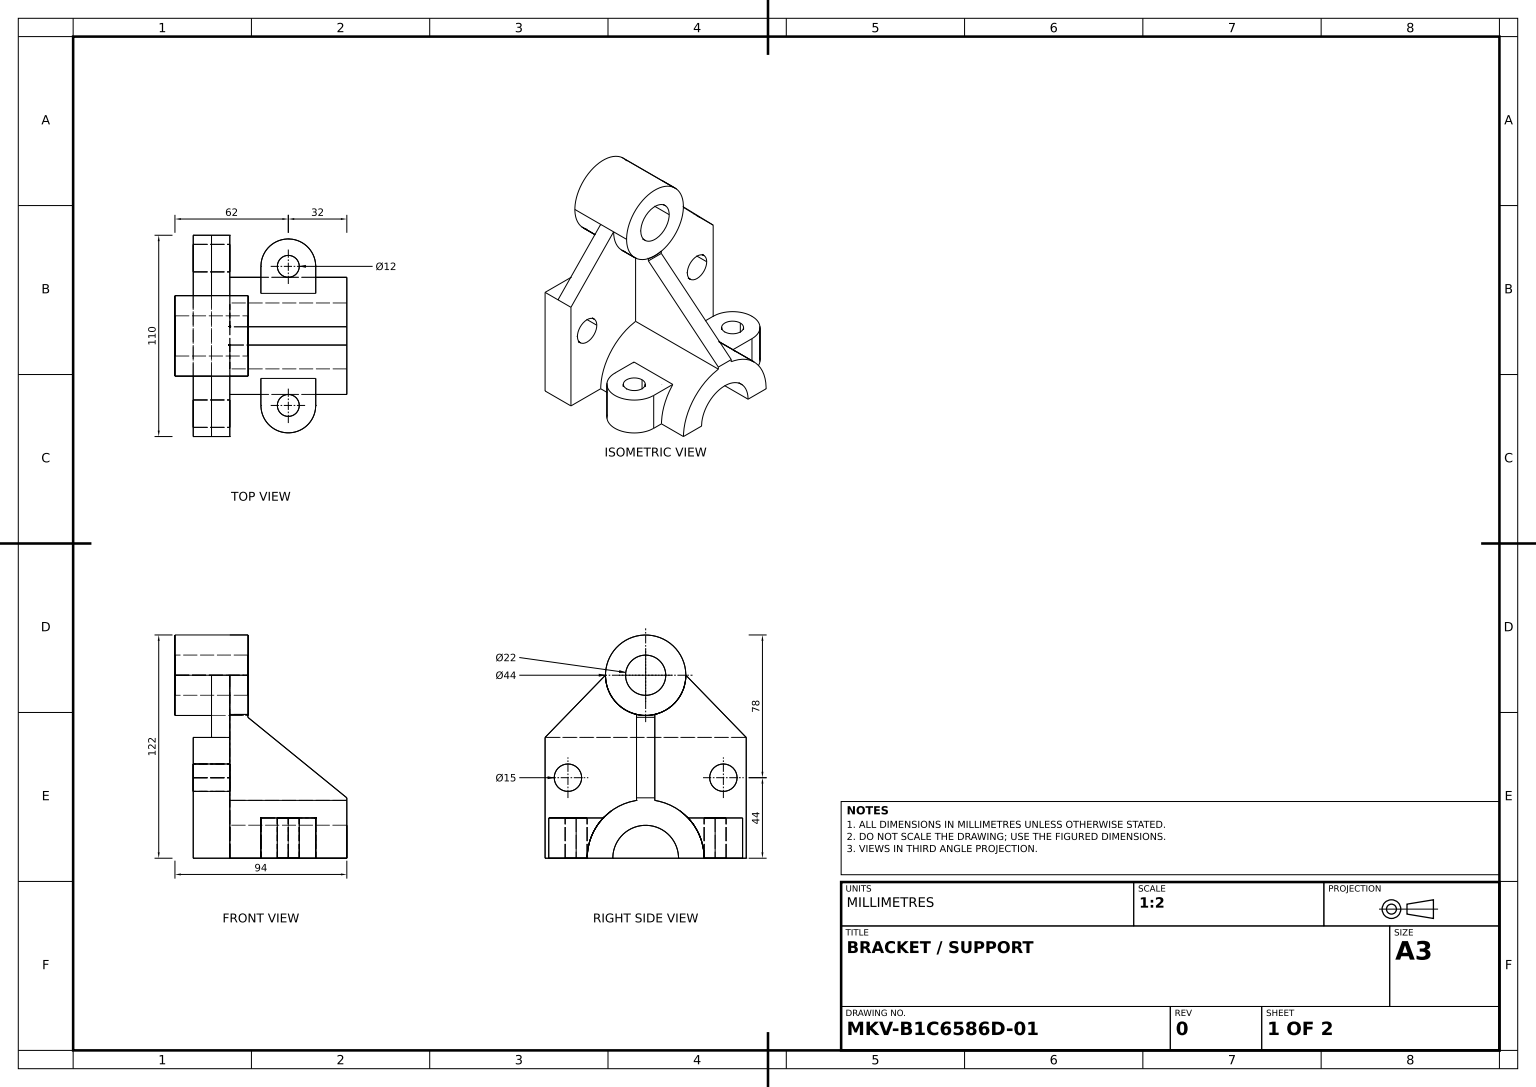
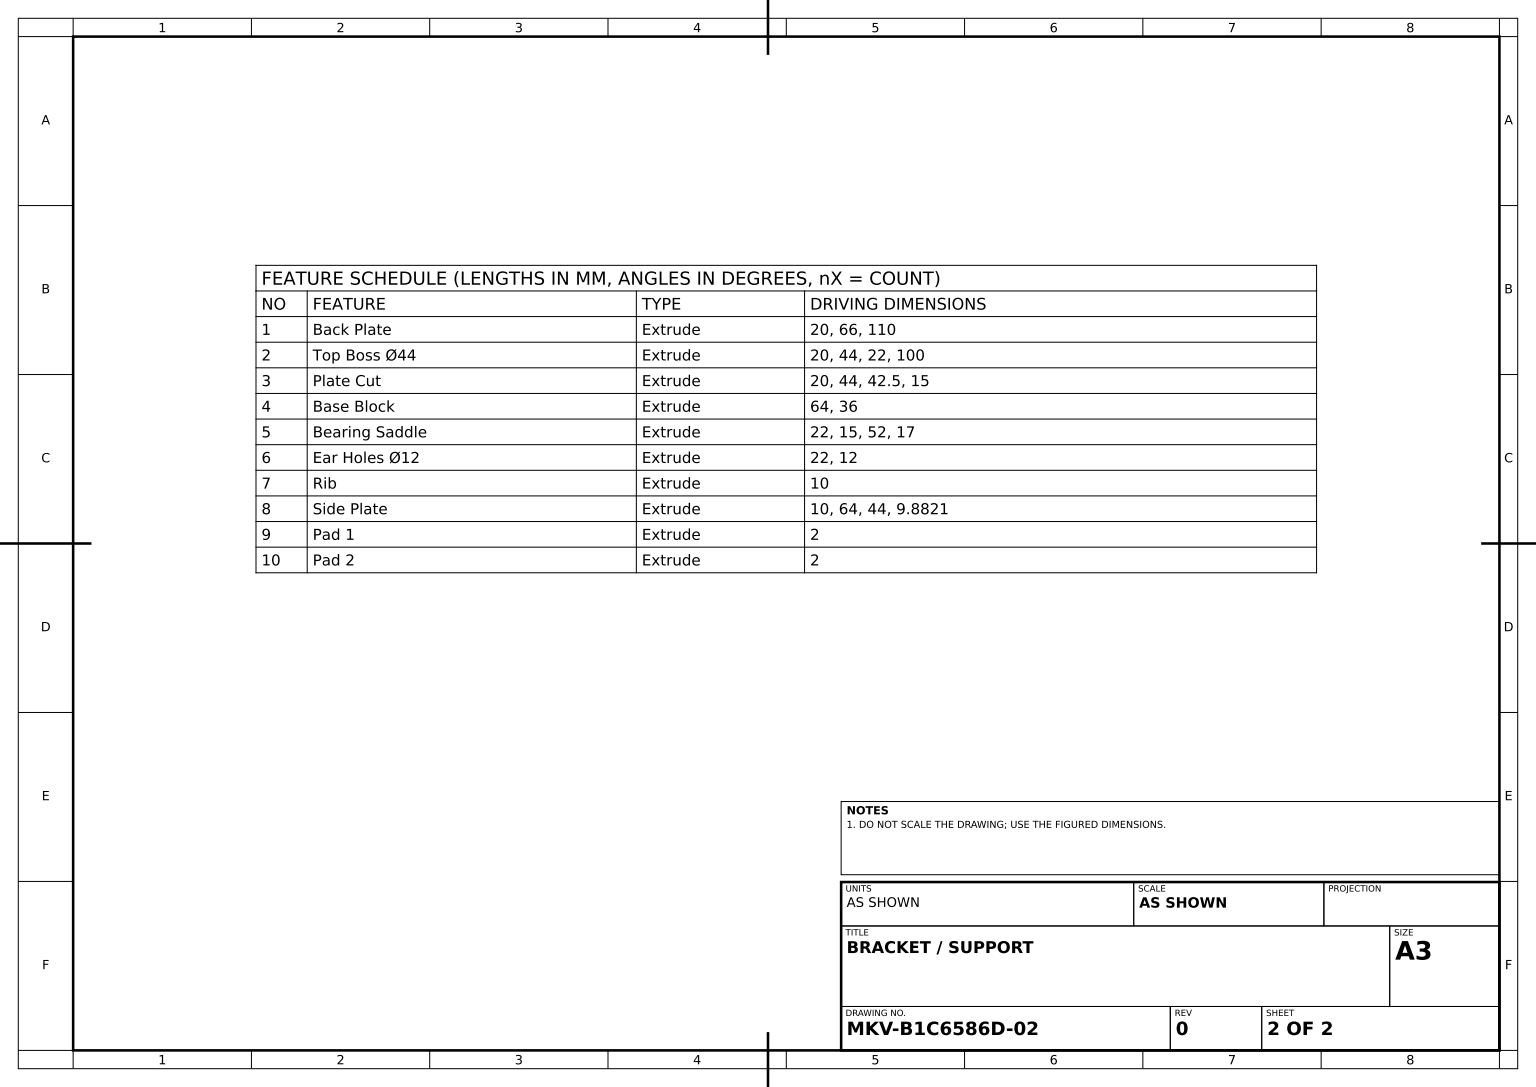
SolidWorks part; units mm, degrees
material "Plain Carbon Steel"
ref_plane "Front Plane" through (0, 0, 0) normal (0, 0, 1) x (1, 0, 0)
ref_plane "Top Plane" through (0, 0, 0) normal (0, 1, 0) x (1, 0, 0)
ref_plane "Right Plane" through (0, 0, 0) normal (1, 0, 0) x (0, 0, -1)
sketch "Back Plate Sketch" plane through (0, 0, 0) normal (1, 0, 0) x (0, 0, -1)
  line L1 (-55, 33) -> (55, 33)
  line L2 (-55, 33) -> (-55, -33)
  line L3 (-55, -33) -> (55, -33)
  line L4 (55, 33) -> (55, -33)
  line L5 (-55, 33) -> (55, -33) construction
  line L6 (-55, -33) -> (55, 33) construction
  point P0 (0, 0)
  dimension "D1" = 66
  dimension "D2" = 110
extrude "Back Plate" add sketch "Back Plate Sketch" along normal mid plane 20
sketch "Top Boss Sketch" plane through (0, 0, 0) normal (1, 0, 0) x (0, 0, -1)
  line L0 (0, -33) -> (0, 67) construction
  line L1 (-55, -33) -> (55, -33) construction
  circle A0 centre (0, 67) radius 22
  circle A1 centre (0, 67) radius 11
  dimension "D1" = 44
  dimension "D2" = 44
  dimension "D3" = 22
  dimension "D4" = 100
extrude "Top Boss Ø44" add sketch "Top Boss Sketch" along normal blind 20 and the other way blind 20 separate body
sketch "Plate Cut Sketch" plane through (10, 0, 0) normal (1, 0, 0) x (0, 0, -1)
  line L0 (0, -33) -> (0, 11) construction
  line L1 (-55, -33) -> (55, -33) construction
  line L2 (0, 11) -> (42.5, 11) construction
  circle A0 centre (42.5, 11) radius 7.5
  circle A1 centre (-42.5, 11) radius 7.5
  dimension "D3" = 15
  dimension "D1" = 44
  dimension "D2" = 42.5
extrude "Plate Cut" cut sketch "Plate Cut Sketch" against normal blind 20
sketch "Base Block Sketch" plane through (10, 0, 0) normal (1, 0, 0) x (0, 0, -1)
  line L0 (-55, -33) -> (55, -33) construction
  line L1 (-32, -33) -> (-18, -33)
  line L2 (18, -33) -> (32, -33)
  arc A0 (32, -33) -> (-32, -33) centre (0, -33) ccw
  arc A1 (18, -33) -> (-18, -33) centre (0, -33) ccw
  dimension "D1" = 64
  dimension "D2" = 36
extrude "Base Block" add sketch "Base Block Sketch" along normal blind 64
sketch "Bearing Saddle Sketch" plane through (0, -33, 0) normal (0, -1, 0) x (1, 0, 0)
  line L0 (42, 38) -> (42, -45.3499) construction
  line L1 (-10, 55) -> (-10, -55) construction
  line L2 (0, 0) -> (88.1033, 0) construction
  line L3 (27, 38) -> (27, 18)
  line L4 (74, 18) -> (10, 18) construction
  line L5 (27, 18) -> (57, 18)
  line L6 (57, 18) -> (57, 38)
  line L7 (27, -38) -> (27, -18)
  line L8 (27, -18) -> (57, -18)
  line L9 (57, -18) -> (57, -38)
  line L10 (10, -55) -> (-10, -55) construction
  arc A3 (27, 38) -> (57, 38) centre (42, 38) cw
  arc A4 (27, -38) -> (57, -38) centre (42, -38) ccw
  dimension "D1" = 15
  dimension "D2" = 52
  dimension "D3" = 17
extrude "Bearing Saddle" add sketch "Bearing Saddle Sketch" against normal blind 22
sketch "Ear Holes Sketch" plane through (0, -11, 0) normal (0, 1, 0) x (1, 0, 0)
  circle A0 centre (42, 38) radius 6
  circle A1 centre (42, -38) radius 6
  dimension "D1" = 12
extrude "Ear Holes Ø12" cut sketch "Ear Holes Sketch" against normal blind 22
sketch "Rib Sketch" plane through (10, 0, 0) normal (1, 0, 0) x (0, 0, -1)
  line L0 (-47.4205, 67) -> (37.9135, 67) construction
  line L1 (-22, 67) -> (-55, 33)
  line L2 (55, 33) -> (22, 67)
  line L5 (32, -33) -> (55, -33)
  line L6 (55, -33) -> (55, 33)
  line L7 (55, 33) -> (-55, 33)
  line L8 (-55, 33) -> (-55, -33)
  line L9 (-55, -33) -> (-32, -33)
  line L12 (55, 33) -> (-55, 33)
  circle A0 centre (0, 67) radius 22 construction
  arc A1 (32, -33) -> (-32, -33) centre (0, -33) ccw
  arc A3 (-22, 67) -> (22, 67) centre (0, 67) ccw
  dimension "D1" = 0
extrude "Rib" add sketch "Rib Sketch" against normal blind 10
sketch "Side Plate Sketch" plane through (0, 0, 0) normal (0, 0, 1) x (1, 0, 0)
  line L1 (10, 44) -> (19.8821, 44)
  line L2 (10, 67) -> (10, 33) construction
  line L3 (10, 44) -> (10, 0)
  line L4 (10, 33) -> (10, -33) construction
  line L5 (10, 0) -> (74, 0)
  line L6 (74, 0) -> (19.8821, 44)
  dimension "D1" = 64
  dimension "D2" = 44
  dimension "D3" = 9.8821
extrude "Side Plate" add sketch "Side Plate Sketch" along normal mid plane 10
sketch "Pad 1 Sketch" plane through (0, 44, 0) normal (0, 1, 0) x (1, 0, 0)
  line L4 (19.8821, 5) -> (10, 5)
  line L5 (10, 5) -> (10, -5)
  line L6 (10, -5) -> (19.8821, -5)
  line L7 (19.8821, -5) -> (19.8821, 5)
  line L8 (19.8821, 5) -> (10, 5)
  line L9 (10, 5) -> (10, -5)
  line L10 (10, -5) -> (19.8821, -5)
  line L11 (19.8821, -5) -> (19.8821, 5)
  dimension "D1" = 0
extrude "Pad 1" add sketch "Pad 1 Sketch" along normal blind 2
sketch "Pad 2 Sketch" plane through (0, 0, 0) normal (0, -1, 0) x (1, 0, 0)
  line L4 (10, -5) -> (74, -5)
  line L5 (74, -5) -> (74, 5)
  line L6 (74, 5) -> (10, 5)
  line L7 (10, 5) -> (10, -5)
  line L8 (10, -5) -> (74, -5)
  line L9 (74, -5) -> (74, 5)
  line L10 (74, 5) -> (10, 5)
  line L11 (10, 5) -> (10, -5)
  dimension "D1" = 0
extrude "Pad 2" add sketch "Pad 2 Sketch" along normal blind 2
